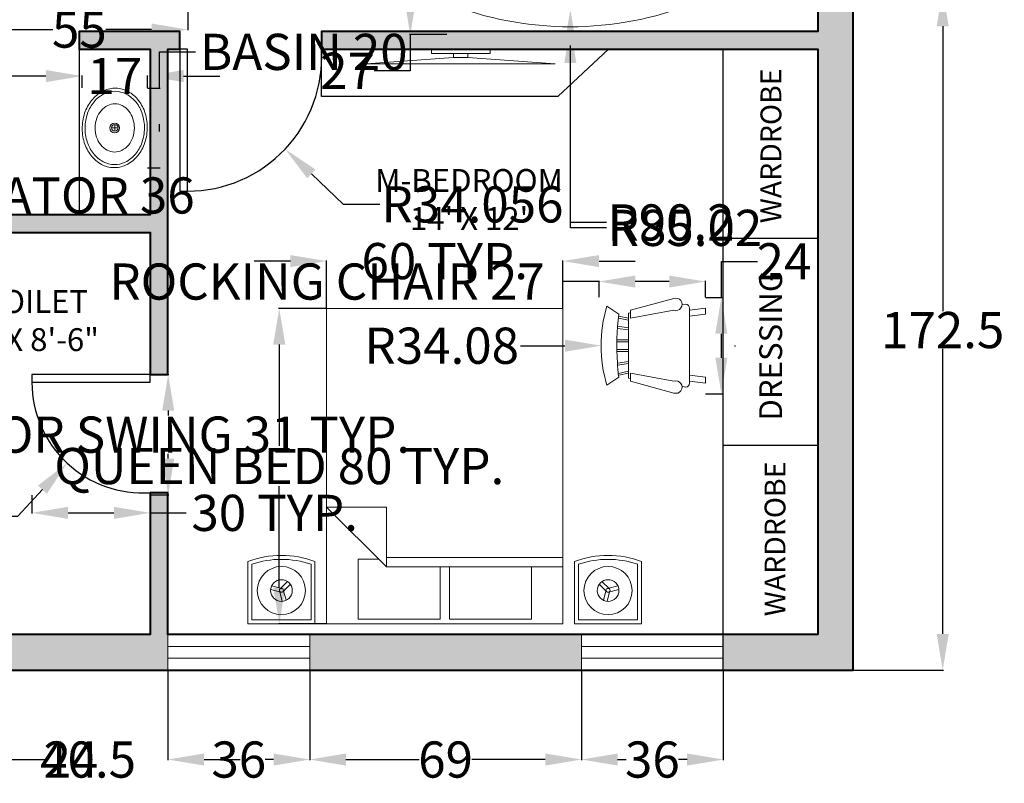
# Model space of a CAD drawing. Units: inches. Extents: x -51 to 563, y -59 to 453.
# Tile 4 of 6: x 211 to 461, y -59 to 134. Entities that reach past the tile are written whole.
import ezdxf

# ---------------------------------------------------------------- set-up
doc = ezdxf.new("R2010")
doc.units = ezdxf.units.IN
doc.header["$MEASUREMENT"] = 0
for name, color, linetype, lineweight in [('A-ANNO-DIMS', 2, 'Continuous', 18), ('A-ANNO-TEXT', 7, 'Continuous', 18), ('A-AREA-IDEN', 7, 'Continuous', 25), ('A-DOOR', 3, 'Continuous', 25), ('A-EQPM', 8, 'Continuous', 18), ('A-FLOR-CASE', 8, 'Continuous', 25), ('A-FLOR-FIXT', 9, 'Continuous', 18), ('A-FURN', 8, 'Continuous', 18), ('A-GLAZ', 4, 'Continuous', 18), ('A-WALL', 7, 'Continuous', 40), ('A-WALL-PATT', 252, 'Continuous', 13)]:
    doc.layers.add(name, color=color, linetype=linetype, lineweight=lineweight)
doc.styles.get("Standard").update_dxf_attribs({"font": 'arial.ttf'})
doc.dimstyles.get("Standard").update_dxf_attribs({"dimtxt": 9.18, "dimasz": 9.18, "dimexe": 0.18, "dimexo": 0.0625, "dimgap": 0.09, "dimtad": 0, "dimtih": 1, "dimtoh": 1, "dimdec": 1, "dimzin": 0, "dimdsep": 46, "dimlunit": 3, "dimtxsty": 'Standard', "dimcen": 0.09, "dimadec": 0, "dimazin": 0, "dimtfac": 1, "dimtdec": 1, "dimtofl": 0, "dimtmove": 0, "dimatfit": 3, "dimfxl": 1, "dimtolj": 1, "dimtzin": 0, "dimarcsym": 0})

# ---------------------------------------------------------------- blocks, each defined once
blk = doc.blocks.new('Bed - Queen')
for p, q in [((0, -80.00003), (0, 0)), ((0, 0), (59.99999, 0)), ((59.99999, 0), (59.99999, -80.00003)), ((7.99999, -1.2), (28.79998, -1.2)), ((7.99999, -14.4), (7.99999, -1.2)), ((28.79998, -1.2), (28.79998, -14.4)), ((31.19999, -1.2), (51.99999, -1.2)), ((31.19999, -14.4), (31.19999, -1.2)), ((51.99999, -1.2), (51.99999, -16.4)), ((0, -14.4), (44.8, -14.4)), ((59.99999, -29.6), (44.8, -14.4)), ((44.8, -14.4), (44.8, -29.6)), ((44.8, -16.8), (0, -16.8)), ((51.99999, -16.4), (46.79936, -16.4)), ((44.8, -29.6), (59.99999, -29.6)), ((59.99999, -80.00003), (0, -80.00003))]:
    blk.add_line(p, q)
blk = doc.blocks.new('Sink - Oval top')
for p, q in [((-1, 0), (1, 0)), ((0, 1), (0, -1))]:
    blk.add_line(p, q)
for points in [[(-12.23, 0.39, 0.117634), (-11.46, -3.36, 0.104469), (-8.88, -6.8, 0.090016), (-5.08, -9.07, 0.08192), (-0.32, -10.02, 0.08192), (4.49, -9.38, 0.090016), (8.42, -7.36, 0.104469), (11.22, -4.09, 0.117634), (12.23, -0.39, 0.117634), (11.46, 3.36, 0.104469), (8.88, 6.8, 0.090016), (5.08, 9.07, 0.08192), (0.32, 10.02, 0.08192), (-4.49, 9.38, 0.090016), (-8.42, 7.36, 0.104469), (-11.22, 4.09, 0.117634)], [(-11.29, 0.16, 0.118622), (-10.52, -3.25, 0.104678), (-8.07, -6.36, 0.089562), (-4.54, -8.37, 0.081185), (-0.13, -9.15, 0.081185), (4.3, -8.49, 0.089562), (7.89, -6.58, 0.104678), (10.42, -3.55, 0.118622), (11.29, -0.16, 0.118622), (10.52, 3.25, 0.104678), (8.07, 6.36, 0.089562), (4.54, 8.37, 0.081185), (0.13, 9.15, 0.081185), (-4.3, 8.49, 0.089562), (-7.89, 6.58, 0.104678), (-10.42, 3.55, 0.118622)], [(-7.42, 0.08, 0.118283), (-6.91, -2.17, 0.104607), (-5.29, -4.21, 0.089718), (-2.97, -5.53, 0.081436), (-0.07, -6.04, 0.081436), (2.84, -5.59, 0.089718), (5.2, -4.33, 0.104607), (6.86, -2.32, 0.118283), (7.42, -0.08, 0.118283), (6.91, 2.17, 0.104607), (5.29, 4.21, 0.089718), (2.97, 5.53, 0.081436), (0.07, 6.04, 0.081436), (-2.84, 5.59, 0.089718), (-5.2, 4.33, 0.104607), (-6.86, 2.32, 0.118283)]]:
    blk.add_lwpolyline(points, format="xyb", close=True)
for radius in [1.5, 1]:
    blk.add_circle((0, 0), radius)
blk = doc.blocks.new('Sofa - Roundback 7 ft.')
for p, q in [((-12.00002, -32.4421), (-12.00003, -6.5971)), ((11.99997, -32.4421), (11.99998, -6.5971)), ((-36.000027, -34), (-36.000027, -11.4696)), ((-35.999844, -13.3819), (35.9998, -13.3819)), ((35.99998, -34), (35.99998, -11.4696)), ((-36.000027, -32.4421), (35.99998, -32.4421))]:
    blk.add_line(p, q)
for points in [[(-36.000027, -34), (-42.000027, -34), (-42.000027, -8)], [(41.99998, -8), (41.99998, -34), (35.99998, -34)]]:
    blk.add_lwpolyline(points)
for centre, radius, start, end in [((0, -114.25), 114.25, 68.43141, 111.5686), ((-0.00001, -127.1968), 121.1968, 72.72033, 107.2797)]:
    blk.add_arc(centre, radius, start, end)
blk = doc.blocks.new('Chair - Rocking')
for p, q in [((-8, -4.5), (-10, -1.5)), ((8, -4.5), (10, -1.5)), ((-7.5, -4.5), (-7, -7)), ((-6.5, -7), (-7.02225, -4.43)), ((-4.5, -7), (-4.96674, -4.19951)), ((-4, -7), (-4.40532, -4.16272)), ((-1.5, -4.05012), (-1.5, -7)), ((-1, -7), (-1, -4.05012)), ((1, -7), (1, -4.04655)), ((1.5, -4.05012), (1.5, -7)), ((4, -7), (4.40187, -4.18694)), ((4.5, -7), (4.96761, -4.19437)), ((6.5, -7), (7, -4.4057)), ((7.5, -4.5), (7, -7)), ((-8.23428, -6.99939), (-8.3093, -7.47958)), ((-8.23041, -7), (8.23915, -7)), ((8.31071, -7.48854), (8.23449, -7.00073)), ((-9, -7.5), (-12, -18.49999)), ((-7, -7.5), (-9, -7.5)), ((-9, -18.49999), (-7, -7.5)), ((7, -7.5), (9, -7.5)), ((9, -18.49999), (7, -7.5)), ((9, -7.5), (12, -18.49999)), ((-10.36644, -20.64523), (-10.5, -21.49999)), ((10.5, -21.49999), (10.3575, -20.58798)), ((-9, -22.49999), (-9.5, -26.49999)), ((0, -22.49999), (-9.5, -22.49999)), ((-8, -26.49999), (-7.5, -22.49999)), ((0, -22.49999), (9.5, -22.49999)), ((8, -26.49999), (7.5, -22.49999)), ((9, -22.49999), (9.5, -26.49999)), ((-9.5, -26.49999), (-8, -26.49999)), ((9.5, -26.49999), (8, -26.49999))]:
    blk.add_line(p, q)
for centre, radius, start, end in [((0, -34.08333), 34.08333, 72.93847, 107.0615), ((0, -68.25004), 64.25, 93.92211, 97.15267), ((0, -68.25004), 64.25, 82.84733, 93.92211), ((-10.5, -18.99999), 1.58114, 161.5651, 18.43495), ((10.5, -18.99999), 1.58114, 161.5651, 18.43495), ((-9.5, -21.49999), 1, 180, 270), ((9.5, -21.49999), 1, 270, 0)]:
    blk.add_arc(centre, radius, start, end)
blk = doc.blocks.new('DR-SWING-30IN')
for p, q in [((30, 30.07), (0, 30.07)), ((0, 30.07), (0, 28.07)), ((30, 28.07), (30, 30.07)), ((0, 28.07), (30, 28.07))]:
    blk.add_line(p, q)
blk.add_arc((28.07, 28.07), 28.07, 180, 273.9499)
blk = doc.blocks.new('TV-FLATSCREEN-48IN')
for p, q in [((0, 0), (22.17, 1.61)), ((48, 0), (25.84, 1.61)), ((0, 0), (48, 0))]:
    blk.add_line(p, q)
for points in [[(16.55, 3.67), (31.46, 3.67), (31.46, 2.61), (16.55, 2.61)], [(22.17, 2.61), (25.84, 2.61), (25.84, 1.61), (22.17, 1.61)]]:
    blk.add_lwpolyline(points, close=True)
blk = doc.blocks.new('*U11')
for p, q in [((-1.31, -0.61), (0.61, 1.31)), ((-0.61, -1.31), (1.31, 0.61))]:
    blk.add_line(p, q)
blk = doc.blocks.new('*U12')
at = {"color": 0, "linetype": 'ByBlock', "lineweight": -2, "transparency": 16777216}
for p, rotation in [((276.07, -10.08), 120), ((277.73, -11.74), 239.9999999999999)]:
    blk.add_blockref('*U11', p, dxfattribs=dict(at, rotation=rotation))
blk.add_blockref('*U11', (278.34, -9.47), dxfattribs=at)
blk = doc.blocks.new('TABLE-SIDE-WITH-LAMP')
for points in [[(17.03, 15.79), (17.03, 0), (0, 0), (0, 15.79, -0.18199)], [(16.03, 15.08), (16.03, 1), (1, 1), (1, 15.08, -0.16668)]]:
    blk.add_lwpolyline(points, format="xyb", close=True)
for centre, radius in [((8.51, 8.42), 6.11), ((8.51, 8.42), 2.75), ((8.51, 8.47), 0.5)]:
    blk.add_circle(centre, radius)
blk.add_blockref('*U12', (-268.87, 18.9))
blk = doc.blocks.new('*D27')
at = {"layer": 'A-ANNO-DIMS', "color": 0, "lineweight": -2, "transparency": 16777216}
for p, q in [((288.78, 61.1), (276.66, 61.1)), ((276.84, 51.92), (276.84, 26.22)), ((276.84, -9.72), (276.84, 15.99)), ((288.78, -18.9), (276.66, -18.9))]:
    blk.add_line(p, q, dxfattribs=at)
at = {"layer": 'A-ANNO-DIMS', "color": 0, "transparency": 16777216}
for points in [[(275.31, 51.92), (278.37, 51.92), (276.84, 61.1)], [(275.31, -9.72), (278.37, -9.72), (276.84, -18.9)]]:
    blk.add_solid(points, dxfattribs=at)
at = {"layer": 'Defpoints', "color": 0, "transparency": 16777216}
for p in [(288.84, 61.1), (276.84, -18.9), (288.84, -18.9)]:
    blk.add_point(p, dxfattribs=at)
at = {"layer": 'A-ANNO-DIMS', "color": 0, "transparency": 16777216, "insert": (276.84, 21.1), "char_height": 9.18, "attachment_point": 5}
blk.add_mtext('\\A1;QUEEN BED 80 TYP.', dxfattribs=at)
blk = doc.blocks.new('*D28')
at = {"layer": 'A-ANNO-DIMS', "color": 0, "lineweight": -2, "transparency": 16777216}
for p, q in [((279.66, 73.1), (270.48, 73.1)), ((288.84, 61.17), (288.84, 73.28)), ((348.84, 61.17), (348.84, 73.28)), ((358.02, 73.1), (367.2, 73.1))]:
    blk.add_line(p, q, dxfattribs=at)
at = {"layer": 'A-ANNO-DIMS', "color": 0, "transparency": 16777216}
for points in [[(279.66, 74.63), (279.66, 71.57), (288.84, 73.1)], [(358.02, 74.63), (358.02, 71.57), (348.84, 73.1)]]:
    blk.add_solid(points, dxfattribs=at)
at = {"layer": 'Defpoints', "color": 0, "transparency": 16777216}
for p in [(288.84, 73.1), (288.84, 61.1), (348.84, 61.1)]:
    blk.add_point(p, dxfattribs=at)
at = {"layer": 'A-ANNO-DIMS', "color": 0, "transparency": 16777216, "insert": (318.84, 73.1), "char_height": 9.18, "attachment_point": 5}
blk.add_mtext('\\A1;60 TYP.', dxfattribs=at)
blk = doc.blocks.new('*D36')
at = {"layer": 'A-ANNO-DIMS', "color": 0, "lineweight": -2, "transparency": 16777216}
for p, q in [((319.42, 157.85), (309.92, 157.85)), ((310.1, 148.67), (310.1, 139.74)), ((319.42, 130.56), (309.92, 130.56)), ((310.1, 130.56), (310.1, 121.38)), ((310.1, 121.38), (300.92, 121.38))]:
    blk.add_line(p, q, dxfattribs=at)
at = {"layer": 'A-ANNO-DIMS', "color": 0, "transparency": 16777216}
for points in [[(308.57, 148.67), (311.63, 148.67), (310.1, 157.85)], [(308.57, 139.74), (311.63, 139.74), (310.1, 130.56)]]:
    blk.add_solid(points, dxfattribs=at)
at = {"layer": 'Defpoints', "color": 0, "transparency": 16777216}
for p in [(319.48, 157.85), (310.1, 130.56), (319.48, 130.56)]:
    blk.add_point(p, dxfattribs=at)
at = {"layer": 'A-ANNO-DIMS', "color": 0, "transparency": 16777216, "insert": (294.18, 121.38), "char_height": 9.18, "attachment_point": 5}
blk.add_mtext('\\A1;27', dxfattribs=at)
blk = doc.blocks.new('*D43')
at = {"layer": 'A-ANNO-DIMS', "color": 0, "lineweight": -2, "transparency": 16777216}
for p, q in [((244.12, 44.35), (248.82, 44.35)), ((248.64, 35.17), (248.64, 33.92)), ((248.64, 22.99), (248.64, 24.24)), ((244.12, 13.81), (248.82, 13.81))]:
    blk.add_line(p, q, dxfattribs=at)
at = {"layer": 'A-ANNO-DIMS', "color": 0, "transparency": 16777216}
for points in [[(247.11, 35.17), (250.17, 35.17), (248.64, 44.35)], [(247.11, 22.99), (250.17, 22.99), (248.64, 13.81)]]:
    blk.add_solid(points, dxfattribs=at)
at = {"layer": 'Defpoints', "color": 0, "transparency": 16777216}
for p in [(244.06, 44.35), (248.64, 44.35), (244.06, 13.81)]:
    blk.add_point(p, dxfattribs=at)
at = {"layer": 'A-ANNO-DIMS', "color": 0, "transparency": 16777216, "insert": (248.64, 29.08), "char_height": 9.18, "attachment_point": 5}
blk.add_mtext('\\A1;DOOR SWING 31 TYP.', dxfattribs=at)
blk = doc.blocks.new('*D44')
at = {"layer": 'A-ANNO-DIMS', "color": 0, "lineweight": -2, "transparency": 16777216}
for p, q in [((214.06, 13.75), (214.06, 9.05)), ((244.06, 13.75), (244.06, 9.05)), ((223.24, 9.23), (234.88, 9.23)), ((244.06, 9.23), (253.24, 9.23))]:
    blk.add_line(p, q, dxfattribs=at)
at = {"layer": 'A-ANNO-DIMS', "color": 0, "transparency": 16777216}
for points in [[(223.24, 10.76), (223.24, 7.7), (214.06, 9.23)], [(234.88, 10.76), (234.88, 7.7), (244.06, 9.23)]]:
    blk.add_solid(points, dxfattribs=at)
at = {"layer": 'Defpoints', "color": 0, "transparency": 16777216}
for p in [(214.06, 13.81), (244.06, 13.81), (244.06, 9.23)]:
    blk.add_point(p, dxfattribs=at)
at = {"layer": 'A-ANNO-DIMS', "color": 0, "transparency": 16777216, "insert": (275.67, 9.23), "char_height": 9.18, "attachment_point": 5}
blk.add_mtext('\\A1;30 TYP.', dxfattribs=at)
blk = doc.blocks.new('*D49')
at = {"layer": 'A-ANNO-DIMS', "color": 0, "lineweight": -2, "transparency": 16777216}
for p, q in [((246.41, 117), (246.41, 126.18)), ((246.41, 126.18), (255.59, 126.18)), ((243.43, 117), (246.59, 117)), ((246.41, 105.95), (246.41, 107.82)), ((243.43, 96.77), (246.59, 96.77))]:
    blk.add_line(p, q, dxfattribs=at)
at = {"layer": 'A-ANNO-DIMS', "color": 0, "transparency": 16777216}
for points in [[(244.88, 107.82), (247.94, 107.82), (246.41, 117)], [(244.88, 105.95), (247.94, 105.95), (246.41, 96.77)]]:
    blk.add_solid(points, dxfattribs=at)
at = {"layer": 'Defpoints', "color": 0, "transparency": 16777216}
for p in [(243.37, 117), (246.41, 117), (243.37, 96.77)]:
    blk.add_point(p, dxfattribs=at)
at = {"layer": 'A-ANNO-DIMS', "color": 0, "transparency": 16777216, "insert": (283.06, 126.18), "char_height": 9.18, "attachment_point": 5}
blk.add_mtext('\\A1;BASIN 20', dxfattribs=at)
blk = doc.blocks.new('*D50')
at = {"layer": 'A-ANNO-DIMS', "color": 0, "lineweight": -2, "transparency": 16777216}
for p, q in [((217.6, 120.04), (208.42, 120.04)), ((226.78, 117.06), (226.78, 120.22)), ((243.37, 117.06), (243.37, 120.22)), ((252.55, 120.04), (261.73, 120.04))]:
    blk.add_line(p, q, dxfattribs=at)
at = {"layer": 'A-ANNO-DIMS', "color": 0, "transparency": 16777216}
for points in [[(217.6, 121.57), (217.6, 118.51), (226.78, 120.04)], [(252.55, 121.57), (252.55, 118.51), (243.37, 120.04)]]:
    blk.add_solid(points, dxfattribs=at)
at = {"layer": 'Defpoints', "color": 0, "transparency": 16777216}
for p in [(226.78, 120.04), (226.78, 117), (243.37, 117)]:
    blk.add_point(p, dxfattribs=at)
at = {"layer": 'A-ANNO-DIMS', "color": 0, "transparency": 16777216, "insert": (235.08, 120.04), "char_height": 9.18, "attachment_point": 5}
blk.add_mtext('\\A1;17', dxfattribs=at)
blk = doc.blocks.new('*D55')
at = {"layer": 'A-ANNO-DIMS', "color": 0, "lineweight": -2, "transparency": 16777216}
for p, q in [((97.59, 95.09), (97.59, 89.57)), ((133.59, 95.09), (133.59, 89.57)), ((106.77, 89.75), (124.41, 89.75)), ((133.59, 89.75), (142.77, 89.75))]:
    blk.add_line(p, q, dxfattribs=at)
at = {"layer": 'A-ANNO-DIMS', "color": 0, "transparency": 16777216}
for points in [[(106.77, 91.28), (106.77, 88.22), (97.59, 89.75)], [(124.41, 91.28), (124.41, 88.22), (133.59, 89.75)]]:
    blk.add_solid(points, dxfattribs=at)
at = {"layer": 'Defpoints', "color": 0, "transparency": 16777216}
for p in [(97.59, 95.15), (133.59, 95.15), (133.59, 89.75)]:
    blk.add_point(p, dxfattribs=at)
at = {"layer": 'A-ANNO-DIMS', "color": 0, "transparency": 16777216, "insert": (201.92, 89.75), "char_height": 9.18, "attachment_point": 5}
blk.add_mtext('\\A1;REFRIGERATOR 36', dxfattribs=at)
blk = doc.blocks.new('*D58')
at = {"layer": 'A-ANNO-DIMS', "color": 0, "lineweight": -2, "transparency": 16777216}
for p, q in [((198.59, 145.43), (198.59, 131.66)), ((253.59, 145.43), (253.59, 131.66)), ((207.77, 131.84), (219.39, 131.84)), ((244.41, 131.84), (232.79, 131.84))]:
    blk.add_line(p, q, dxfattribs=at)
at = {"layer": 'A-ANNO-DIMS', "color": 0, "transparency": 16777216}
for points in [[(207.77, 133.37), (207.77, 130.31), (198.59, 131.84)], [(244.41, 133.37), (244.41, 130.31), (253.59, 131.84)]]:
    blk.add_solid(points, dxfattribs=at)
at = {"layer": 'Defpoints', "color": 0, "transparency": 16777216}
for p in [(198.59, 145.49), (253.59, 145.49), (253.59, 131.84)]:
    blk.add_point(p, dxfattribs=at)
at = {"layer": 'A-ANNO-DIMS', "color": 0, "transparency": 16777216, "insert": (226.09, 131.84), "char_height": 9.18, "attachment_point": 5}
blk.add_mtext('\\A1;55', dxfattribs=at)
blk = doc.blocks.new('*D63')
at = {"layer": 'A-ANNO-DIMS', "color": 0, "lineweight": -2, "transparency": 16777216}
for p, q in [((358.02, 67.91), (348.84, 67.91)), ((358.02, 63.92), (358.02, 68.09)), ((375.84, 67.91), (367.2, 67.91)), ((385.02, 63.92), (385.02, 68.09))]:
    blk.add_line(p, q, dxfattribs=at)
at = {"layer": 'A-ANNO-DIMS', "color": 0, "transparency": 16777216}
for points in [[(367.2, 69.44), (367.2, 66.38), (358.02, 67.91)], [(375.84, 69.44), (375.84, 66.38), (385.02, 67.91)]]:
    blk.add_solid(points, dxfattribs=at)
at = {"layer": 'Defpoints', "color": 0, "transparency": 16777216}
for p in [(358.02, 67.91), (358.02, 63.86), (385.02, 63.86)]:
    blk.add_point(p, dxfattribs=at)
at = {"layer": 'A-ANNO-DIMS', "color": 0, "transparency": 16777216, "insert": (288.97, 67.91), "char_height": 9.18, "attachment_point": 5}
blk.add_mtext('\\A1;ROCKING CHAIR 27', dxfattribs=at)
blk = doc.blocks.new('*D64')
at = {"layer": 'A-ANNO-DIMS', "color": 0, "lineweight": -2, "transparency": 16777216}
for p, q in [((389.07, 63.86), (389.07, 73.04)), ((389.07, 73.04), (398.25, 73.04)), ((385.08, 63.86), (389.25, 63.86)), ((389.07, 48.6), (389.07, 54.68)), ((385.08, 39.42), (389.25, 39.42))]:
    blk.add_line(p, q, dxfattribs=at)
at = {"layer": 'A-ANNO-DIMS', "color": 0, "transparency": 16777216}
for points in [[(387.54, 54.68), (390.6, 54.68), (389.07, 63.86)], [(387.54, 48.6), (390.6, 48.6), (389.07, 39.42)]]:
    blk.add_solid(points, dxfattribs=at)
at = {"layer": 'Defpoints', "color": 0, "transparency": 16777216}
for p in [(385.02, 63.86), (389.07, 63.86), (385.02, 39.42)]:
    blk.add_point(p, dxfattribs=at)
at = {"layer": 'A-ANNO-DIMS', "color": 0, "transparency": 16777216, "insert": (404.97, 73.04), "char_height": 9.18, "attachment_point": 5}
blk.add_mtext('\\A1;24', dxfattribs=at)
blk = doc.blocks.new('*D72')
at = {"layer": 'A-ANNO-DIMS', "color": 0, "lineweight": -2, "transparency": 16777216}
for p, q in [((422.62, 141.85), (445.44, 141.85)), ((445.26, 132.67), (445.26, 60.37)), ((445.26, -21.47), (445.26, 50.82)), ((422.62, -30.65), (445.44, -30.65))]:
    blk.add_line(p, q, dxfattribs=at)
at = {"layer": 'A-ANNO-DIMS', "color": 0, "transparency": 16777216}
for points in [[(443.73, 132.67), (446.79, 132.67), (445.26, 141.85)], [(443.73, -21.47), (446.79, -21.47), (445.26, -30.65)]]:
    blk.add_solid(points, dxfattribs=at)
at = {"layer": 'Defpoints', "color": 0, "transparency": 16777216}
for p in [(422.56, 141.85), (422.56, -30.65), (445.26, -30.65)]:
    blk.add_point(p, dxfattribs=at)
at = {"layer": 'A-ANNO-DIMS', "color": 0, "transparency": 16777216, "insert": (445.26, 55.6), "char_height": 9.18, "attachment_point": 5}
blk.add_mtext('\\A1;172.5', dxfattribs=at)
blk = doc.blocks.new('*D76')
at = {"layer": 'A-ANNO-DIMS', "color": 0, "lineweight": -2, "transparency": 16777216}
for p, q in [((184.06, -30.71), (184.06, -53.53)), ((208.06, -30.71), (208.06, -53.53)), ((193.24, -53.35), (198.88, -53.35)), ((208.06, -53.35), (217.24, -53.35))]:
    blk.add_line(p, q, dxfattribs=at)
at = {"layer": 'A-ANNO-DIMS', "color": 0, "transparency": 16777216}
for points in [[(193.24, -51.82), (193.24, -54.88), (184.06, -53.35)], [(198.88, -51.82), (198.88, -54.88), (208.06, -53.35)]]:
    blk.add_solid(points, dxfattribs=at)
at = {"layer": 'Defpoints', "color": 0, "transparency": 16777216}
for p in [(184.06, -30.65), (208.06, -30.65), (208.06, -53.35)]:
    blk.add_point(p, dxfattribs=at)
at = {"layer": 'A-ANNO-DIMS', "color": 0, "transparency": 16777216, "insert": (223.96, -53.35), "char_height": 9.18, "attachment_point": 5}
blk.add_mtext('\\A1;24', dxfattribs=at)
blk = doc.blocks.new('*D77')
at = {"layer": 'A-ANNO-DIMS', "color": 0, "lineweight": -2, "transparency": 16777216}
for p, q in [((208.058368, -30.714601), (208.058368, -53.532101)), ((248.558368, -30.714601), (248.558368, -53.532101)), ((198.878368, -53.352101), (189.698368, -53.352101)), ((257.738368, -53.352101), (266.918368, -53.352101))]:
    blk.add_line(p, q, dxfattribs=at)
at = {"layer": 'A-ANNO-DIMS', "color": 0, "transparency": 16777216}
for points in [[(198.878368, -51.822101), (198.878368, -54.882101), (208.058368, -53.352101)], [(257.738368, -51.822101), (257.738368, -54.882101), (248.558368, -53.352101)]]:
    blk.add_solid(points, dxfattribs=at)
at = {"layer": 'Defpoints', "color": 0, "transparency": 16777216}
for p in [(208.058368, -30.652101), (248.558368, -30.652101), (248.558368, -53.352101)]:
    blk.add_point(p, dxfattribs=at)
at = {"layer": 'A-ANNO-DIMS', "color": 0, "transparency": 16777216, "insert": (228.308368, -53.352101), "char_height": 9.18, "attachment_point": 5}
blk.add_mtext('\\A1;40.5', dxfattribs=at)
blk = doc.blocks.new('*D78')
at = {"layer": 'A-ANNO-DIMS', "color": 0, "lineweight": -2, "transparency": 16777216}
for p, q in [((248.56, -30.71), (248.56, -53.53)), ((284.56, -30.71), (284.56, -53.53)), ((257.74, -53.35), (259.9, -53.35)), ((275.38, -53.35), (273.22, -53.35))]:
    blk.add_line(p, q, dxfattribs=at)
at = {"layer": 'A-ANNO-DIMS', "color": 0, "transparency": 16777216}
for points in [[(257.74, -51.82), (257.74, -54.88), (248.56, -53.35)], [(275.38, -51.82), (275.38, -54.88), (284.56, -53.35)]]:
    blk.add_solid(points, dxfattribs=at)
at = {"layer": 'Defpoints', "color": 0, "transparency": 16777216}
for p in [(248.56, -30.65), (284.56, -30.65), (284.56, -53.35)]:
    blk.add_point(p, dxfattribs=at)
at = {"layer": 'A-ANNO-DIMS', "color": 0, "transparency": 16777216, "insert": (266.56, -53.35), "char_height": 9.18, "attachment_point": 5}
blk.add_mtext('\\A1;36', dxfattribs=at)
blk = doc.blocks.new('*D79')
at = {"layer": 'A-ANNO-DIMS', "color": 0, "lineweight": -2, "transparency": 16777216}
for p, q in [((284.56, -30.71), (284.56, -53.53)), ((353.56, -30.71), (353.56, -53.53)), ((293.74, -53.35), (312.36, -53.35)), ((344.38, -53.35), (325.76, -53.35))]:
    blk.add_line(p, q, dxfattribs=at)
at = {"layer": 'A-ANNO-DIMS', "color": 0, "transparency": 16777216}
for points in [[(293.74, -51.82), (293.74, -54.88), (284.56, -53.35)], [(344.38, -51.82), (344.38, -54.88), (353.56, -53.35)]]:
    blk.add_solid(points, dxfattribs=at)
at = {"layer": 'Defpoints', "color": 0, "transparency": 16777216}
for p in [(284.56, -30.65), (353.56, -30.65), (353.56, -53.35)]:
    blk.add_point(p, dxfattribs=at)
at = {"layer": 'A-ANNO-DIMS', "color": 0, "transparency": 16777216, "insert": (319.06, -53.35), "char_height": 9.18, "attachment_point": 5}
blk.add_mtext('\\A1;69', dxfattribs=at)
blk = doc.blocks.new('*D80')
at = {"layer": 'A-ANNO-DIMS', "color": 0, "lineweight": -2, "transparency": 16777216}
for p, q in [((353.56, -30.71), (353.56, -53.53)), ((389.56, -30.71), (389.56, -53.53)), ((362.74, -53.35), (364.9, -53.35)), ((380.38, -53.35), (378.22, -53.35))]:
    blk.add_line(p, q, dxfattribs=at)
at = {"layer": 'A-ANNO-DIMS', "color": 0, "transparency": 16777216}
for points in [[(362.74, -51.82), (362.74, -54.88), (353.56, -53.35)], [(380.38, -51.82), (380.38, -54.88), (389.56, -53.35)]]:
    blk.add_solid(points, dxfattribs=at)
at = {"layer": 'Defpoints', "color": 0, "transparency": 16777216}
for p in [(353.56, -30.65), (389.56, -30.65), (389.56, -53.35)]:
    blk.add_point(p, dxfattribs=at)
at = {"layer": 'A-ANNO-DIMS', "color": 0, "transparency": 16777216, "insert": (371.56, -53.35), "char_height": 9.18, "attachment_point": 5}
blk.add_mtext('\\A1;36', dxfattribs=at)
blk = doc.blocks.new('*D82')
at = {"layer": 'A-ANNO-DIMS', "color": 0, "lineweight": -2, "transparency": 16777216}
for p, q in [((253.56, 124.81), (253.56, 124.99)), ((253.47, 124.9), (253.65, 124.9)), ((293.17, 87.49), (284.99, 95.22)), ((302.35, 87.49), (293.17, 87.49))]:
    blk.add_line(p, q, dxfattribs=at)
at = {"layer": 'A-ANNO-DIMS', "color": 0, "transparency": 16777216}
blk.add_solid([(286.04, 96.33), (283.94, 94.1), (278.32, 101.52)], dxfattribs=at)
at = {"layer": 'Defpoints', "color": 0, "transparency": 16777216}
for p in [(253.56, 124.9), (278.32, 101.52)]:
    blk.add_point(p, dxfattribs=at)
at = {"layer": 'A-ANNO-DIMS', "color": 0, "transparency": 16777216, "insert": (325.89, 87.49), "char_height": 9.18, "attachment_point": 5}
blk.add_mtext('\\A1;R34.056', dxfattribs=at)
blk = doc.blocks.new('*D85')
at = {"layer": 'A-ANNO-DIMS', "color": 0, "lineweight": -2, "transparency": 16777216}
for p, q in [((242.04, 42.35), (242.22, 42.35)), ((242.13, 42.26), (242.13, 42.44)), ((210.45, 8.41), (216.71, 15.12)), ((201.27, 8.41), (210.45, 8.41))]:
    blk.add_line(p, q, dxfattribs=at)
at = {"layer": 'A-ANNO-DIMS', "color": 0, "transparency": 16777216}
blk.add_solid([(215.59, 16.16), (217.83, 14.07), (222.97, 21.83)], dxfattribs=at)
at = {"layer": 'Defpoints', "color": 0, "transparency": 16777216}
for p in [(242.13, 42.35), (222.97, 21.83)]:
    blk.add_point(p, dxfattribs=at)
at = {"layer": 'A-ANNO-DIMS', "color": 0, "transparency": 16777216, "insert": (167.79, 8.41), "char_height": 9.18, "attachment_point": 5}
blk.add_mtext('\\A1;2X R28.067', dxfattribs=at)
blk = doc.blocks.new('*D91')
at = {"layer": 'A-ANNO-DIMS', "color": 0, "lineweight": -2, "transparency": 16777216}
for p, q in [((350.65, 227.21), (350.83, 227.21)), ((350.74, 227.12), (350.74, 227.3)), ((350.74, 82.9), (350.74, 127.83)), ((359.92, 82.9), (350.74, 82.9))]:
    blk.add_line(p, q, dxfattribs=at)
at = {"layer": 'A-ANNO-DIMS', "color": 0, "transparency": 16777216}
blk.add_solid([(352.27, 127.83), (349.21, 127.83), (350.74, 137.01)], dxfattribs=at)
at = {"layer": 'Defpoints', "color": 0, "transparency": 16777216}
for p in [(350.74, 227.21), (350.74, 137.01)]:
    blk.add_point(p, dxfattribs=at)
at = {"layer": 'A-ANNO-DIMS', "color": 0, "transparency": 16777216, "insert": (376.27, 82.9), "char_height": 9.18, "attachment_point": 5}
blk.add_mtext('\\A1;R90.2', dxfattribs=at)
blk = doc.blocks.new('*D92')
at = {"layer": 'A-ANNO-DIMS', "color": 0, "lineweight": -2, "transparency": 16777216}
for p, q in [((350.65, 217.57), (350.83, 217.57)), ((350.74, 217.48), (350.74, 217.66)), ((350.74, 81.53), (350.74, 123.37)), ((359.92, 81.53), (350.74, 81.53))]:
    blk.add_line(p, q, dxfattribs=at)
at = {"layer": 'A-ANNO-DIMS', "color": 0, "transparency": 16777216}
blk.add_solid([(352.27, 123.37), (349.21, 123.37), (350.74, 132.55)], dxfattribs=at)
at = {"layer": 'Defpoints', "color": 0, "transparency": 16777216}
for p in [(350.74, 217.57), (350.74, 132.55)]:
    blk.add_point(p, dxfattribs=at)
at = {"layer": 'A-ANNO-DIMS', "color": 0, "transparency": 16777216, "insert": (379.84, 81.53), "char_height": 9.18, "attachment_point": 5}
blk.add_mtext('\\A1;R85.02', dxfattribs=at)
blk = doc.blocks.new('*D97')
at = {"layer": 'A-ANNO-DIMS', "color": 0, "lineweight": -2, "transparency": 16777216}
for p, q in [((338.07, 51.64), (349.34, 51.64)), ((392.51, 51.64), (392.69, 51.64)), ((392.6, 51.55), (392.6, 51.73))]:
    blk.add_line(p, q, dxfattribs=at)
at = {"layer": 'A-ANNO-DIMS', "color": 0, "transparency": 16777216}
blk.add_solid([(349.34, 53.17), (349.34, 50.11), (358.52, 51.64)], dxfattribs=at)
at = {"layer": 'Defpoints', "color": 0, "transparency": 16777216}
for p in [(358.52, 51.64), (392.6, 51.64)]:
    blk.add_point(p, dxfattribs=at)
at = {"layer": 'A-ANNO-DIMS', "color": 0, "transparency": 16777216, "insert": (318.09, 51.64), "char_height": 9.18, "attachment_point": 5}
blk.add_mtext('\\A1;R34.08', dxfattribs=at)

msp = doc.modelspace()

# ---------------------------------------------------------------- linework, layer by layer
at = {"layer": 'A-DOOR'}
for p, q in [((251.5584, 126.8479), (251.5584, 90.8479)), ((253.5584, 126.8479), (251.5584, 126.8479)), ((253.5584, 90.8479), (253.5584, 126.8479)), ((251.5584, 90.8479), (253.5584, 90.8479))]:
    msp.add_line(p, q, dxfattribs=at)
msp.add_arc((253.5584, 124.9035), 34.0556, 270, 3.273154, dxfattribs=at)
at = {"layer": 'A-FLOR-CASE'}
for p, q in [((226.0584, 126.8479), (226.0584, 84.8479)), ((287.5584, 114.8479), (287.5584, 126.8479)), ((347.5584, 114.8479), (360.3831, 126.8479)), ((389.5584, -30.6521), (389.5584, 126.8479))]:
    msp.add_line(p, q, dxfattribs=at)
for points in [[(347.5584, 114.8479), (287.5584, 114.8479)], [(413.5584, 78.8479), (389.5584, 78.8479)], [(413.5584, 26.3479), (389.5584, 26.3479)]]:
    msp.add_lwpolyline(points, dxfattribs=at)
at = {"layer": 'A-GLAZ'}
for p, q in [((248.5584, -21.6521), (248.5584, -30.6521)), ((284.5584, -21.6521), (284.5584, -30.6521)), ((353.5584, -30.6521), (353.5584, -21.6521))]:
    msp.add_line(p, q, dxfattribs=at)
for points in [[(284.5584, -24.6521), (248.5584, -24.6521)], [(389.5584, -24.6521), (353.5584, -24.6521)], [(284.5584, -27.6521), (248.5584, -27.6521)], [(389.5584, -27.6521), (353.5584, -27.6521)]]:
    msp.add_lwpolyline(points, dxfattribs=at)
at = {"layer": 'A-WALL'}
for points in [[(35.5584, -30.6521), (284.5584, -30.6521), (413.5584, -30.6521), (422.5584, -30.6521), (422.5584, 0.8479), (422.5584, 200.3479), (413.5584, 200.3479), (413.5584, 131.3479), (287.5584, 131.3479), (287.5584, 126.8479), (413.5584, 126.8479), (413.5584, -21.6521), (284.5584, -21.6521), (248.5584, -21.6521), (248.5584, 14.3479), (244.0584, 14.3479), (244.0584, -21.6521), (184.0584, -21.6521)], [(184.0584, 80.3479), (244.0584, 80.3479), (244.0584, 44.3479), (248.5584, 44.3479), (248.5584, 126.8479), (251.5584, 126.8479), (251.5584, 131.3479), (226.0584, 131.3479), (226.0584, 126.8479), (244.0584, 126.8479), (244.0584, 84.8479), (179.5584, 84.8479)]]:
    msp.add_lwpolyline(points, dxfattribs=at)
at = {"layer": 'A-WALL-PATT'}
for points in [[(413.5584, -21.6521), (422.5584, -30.6521), (413.5584, 141.8479), (422.5584, 141.8479)], [(251.5584, 126.8479), (251.5584, 131.3479), (226.0584, 126.8479), (226.0584, 131.3479)], [(244.0584, 126.8479), (248.5584, 126.8479), (251.5584, 126.8479), (251.5584, 131.3479)], [(413.5584, 126.8479), (413.5584, 131.3479), (287.5584, 126.8479), (287.5584, 131.3479)], [(244.0584, 44.3479), (248.5584, 44.3479), (244.0584, 126.8479), (248.5584, 126.8479)], [(184.0584, 80.3479), (179.5584, 84.8479), (244.0584, 80.3479), (244.0584, 84.8479)], [(244.0584, 80.3479), (244.0584, 84.8479), (244.0584, 44.3479), (248.5584, 44.3479)], [(244.0584, -21.6521), (248.5584, -30.6521), (244.0584, 14.3479), (248.5584, 14.3479)], [(208.0584, -21.6521), (208.0584, -30.6521), (244.0584, -21.6521), (248.5584, -30.6521)], [(284.5584, -21.6521), (284.5584, -30.6521), (353.5584, -21.6521), (353.5584, -30.6521)], [(389.5584, -21.6521), (389.5584, -30.6521), (413.5584, -21.6521), (422.5584, -30.6521)]]:
    msp.add_solid(points, dxfattribs=at)

# ---------------------------------------------------------------- block references
at = {"layer": 'A-DOOR'}
msp.add_blockref('DR-SWING-30IN', (214.058, 14.282), dxfattribs=at)
at = {"layer": 'A-EQPM'}
msp.add_blockref('TV-FLATSCREEN-48IN', (298.907, 123.175), dxfattribs=at)
at = {"layer": 'A-FLOR-FIXT', "xscale": 0.8240563005509539, "yscale": 0.8240563005509539, "zscale": 0.8240563005509539, "rotation": 90}
msp.add_blockref('Sink - Oval top', (235.0754, 106.8861), dxfattribs=at)
at = {"layer": 'A-FURN', "xscale": 0.7442004743752547, "yscale": 0.7442004743752547, "zscale": 0.7442004743752547, "rotation": 180}
msp.add_blockref('Sofa - Roundback 7 ft.', (350.7357, 132.5493), dxfattribs=at)
at = {"layer": 'A-FURN'}
for name, p, rotation in [('Chair - Rocking', (358.5179, 51.6377), 90), ('Bed - Queen', (348.8436, -18.8966), 180)]:
    msp.add_blockref(name, p, dxfattribs=dict(at, rotation=rotation))
msp.add_blockref('TABLE-SIDE-WITH-LAMP', (268.87, -18.897), dxfattribs=at)
at = {"layer": 'A-FURN', "extrusion": (0, 0, -1), "zscale": -1}
msp.add_blockref('TABLE-SIDE-WITH-LAMP', (-368.8172, -18.897), dxfattribs=at)

# ---------------------------------------------------------------- texts
at = {"layer": 'A-ANNO-TEXT', "char_height": 5.298513, "attachment_point": 1, "rotation": 90}
for insert in [(398.9999, 79.6901), (400.0507, -20.0339)]:
    msp.add_mtext_dynamic_manual_height_columns('\\pxqc;WARDROBE', width=45.301277, gutter_width=0.9135, heights=[0], dxfattribs=dict(at, insert=insert))
at = {"layer": 'A-AREA-IDEN', "char_height": 5.8, "attachment_point": 1}
for s, insert in [("\\pxqc;M-BEDROOM\\P14' X 12'", (300.2312, 96.454)), ('\\pxqc;TOILET\\P5\' X 8\'-6"', (190.204, 65.7447))]:
    msp.add_mtext_dynamic_manual_height_columns(s, width=49.588896, gutter_width=1, heights=[0], dxfattribs=dict(at, insert=insert))
at = {"layer": 'A-AREA-IDEN', "insert": (398.6913, 29.7461), "char_height": 5.8, "attachment_point": 1, "rotation": 90}
msp.add_mtext_dynamic_manual_height_columns('\\pxqc;DRESSING', width=43.815721, gutter_width=1, heights=[0], dxfattribs=at)

# ---------------------------------------------------------------- dimensions: what is measured, and where the dimension line sits
at = {"layer": 'A-ANNO-DIMS'}
for center, mpoint, override, picture, middle in [((350.7357, 227.2092), (350.736, 137.0145), {"dimdec": 1, "dimlfac": 1, "dimrnd": 0, "dimzin": 0, "dimdsep": 46, "dimlunit": 2}, '*D91', (376.2747, 82.8976)), ((350.7357, 217.5742), (350.736, 132.5493), {"dimdec": 2, "dimlfac": 1, "dimrnd": 0, "dimzin": 0, "dimdsep": 46, "dimlunit": 2}, '*D92', (379.8409, 81.5343)), ((253.5584, 124.9035), (278.3171, 101.5199), {"dimdec": 3, "dimlfac": 1, "dimrnd": 0, "dimzin": 0, "dimdsep": 46, "dimlunit": 2}, '*D82', (325.887, 87.4898)), ((392.6012, 51.6377), (358.5179, 51.638), {"dimdec": 2, "dimlfac": 1, "dimrnd": 0, "dimzin": 0, "dimdsep": 46, "dimlunit": 2}, '*D97', (338.0679, 51.6382))]:
    dim = msp.add_radius_dim(center=center, mpoint=mpoint, dimstyle='Standard', override=override, dxfattribs=at)
    dim.commit()
    dim.dimension.update_dxf_attribs({"geometry": picture, "text_midpoint": middle, "dimtype": 164})
for base, p1, p2, angle, override, picture, middle in [((310.1023, 130.5647), (319.4793, 157.8521), (319.4793, 130.5647), 270, {"dimdec": 0, "dimlfac": 1, "dimrnd": 0, "dimzin": 0, "dimdsep": 46, "dimlunit": 2}, '*D36', (294.179, 121.3847)), ((445.2584, -30.6521), (422.5584, 141.8479), (422.5584, -30.6521), 90, {"dimdec": 1, "dimlfac": 1, "dimrnd": 0, "dimzin": 0, "dimdsep": 46, "dimlunit": 2}, '*D72', (445.2584, 55.5979)), ((226.7786, 120.0365), (243.3723, 117.0018), (226.7786, 117.0018), 180, {"dimdec": 0, "dimlfac": 1, "dimrnd": 0, "dimzin": 0, "dimdsep": 46, "dimlunit": 2}, '*D50', (235.0754, 120.0365)), ((389.0679, 63.8552), (385.0179, 39.4201), (385.0179, 63.8552), 90, {"dimdec": 0, "dimlfac": 1, "dimrnd": 0, "dimzin": 0, "dimdsep": 46, "dimlunit": 2}, '*D64', (404.9724, 73.0352))]:
    dim = msp.add_linear_dim(base=base, p1=p1, p2=p2, angle=angle, dimstyle='Standard', override=override, dxfattribs=at)
    dim.commit()
    dim.dimension.update_dxf_attribs({"geometry": picture, "text_midpoint": middle})
for base, p1, p2, override, picture, middle in [((253.5874, 131.838), (198.5874, 145.488), (253.5874, 145.488), {"dimdec": 0, "dimlfac": 1, "dimrnd": 0, "dimzin": 0, "dimdsep": 46, "dimlunit": 2}, '*D58', (226.0874, 131.838)), ((208.0584, -53.3521), (184.0584, -30.6521), (208.0584, -30.6521), {"dimdec": 0, "dimlfac": 1, "dimrnd": 0, "dimzin": 0, "dimdsep": 46, "dimlunit": 2}, '*D76', (223.9629, -53.3521)), ((248.5584, -53.3521), (208.0584, -30.6521), (248.5584, -30.6521), {"dimdec": 1, "dimlfac": 1, "dimrnd": 0, "dimzin": 0, "dimdsep": 46, "dimlunit": 2}, '*D77', (228.3084, -53.3521)), ((284.5584, -53.3521), (248.5584, -30.6521), (284.5584, -30.6521), {"dimdec": 0, "dimlfac": 1, "dimrnd": 0, "dimzin": 0, "dimdsep": 46, "dimlunit": 2}, '*D78', (266.5584, -53.3521)), ((353.5584, -53.3521), (284.5584, -30.6521), (353.5584, -30.6521), {"dimdec": 0, "dimlfac": 1, "dimrnd": 0, "dimzin": 0, "dimdsep": 46, "dimlunit": 2}, '*D79', (319.0584, -53.3521)), ((389.5584, -53.3521), (353.5584, -30.6521), (389.5584, -30.6521), {"dimdec": 0, "dimlfac": 1, "dimrnd": 0, "dimzin": 0, "dimdsep": 46, "dimlunit": 2}, '*D80', (371.5584, -53.3521))]:
    dim = msp.add_linear_dim(base=base, p1=p1, p2=p2, dimstyle='Standard', override=override, dxfattribs=at)
    dim.commit()
    dim.dimension.update_dxf_attribs({"geometry": picture, "text_midpoint": middle})
for base, p1, p2, angle, text, picture, middle in [((246.407, 117.0018), (243.3723, 96.7705), (243.3723, 117.0018), 90, 'BASIN <>', '*D49', (283.0573, 126.1818)), ((358.0179, 67.9052), (385.0179, 63.8552), (358.0179, 63.8552), 180, 'ROCKING CHAIR <>', '*D63', (288.9715, 67.9052)), ((288.8436, 73.1034), (348.8436, 61.1034), (288.8436, 61.1034), 180, '<> TYP.', '*D28', (318.8436, 73.1034)), ((276.8436, -18.8966), (288.8436, 61.1034), (288.8436, -18.8966), 270, 'QUEEN BED <> TYP.', '*D27', (276.8436, 21.1034)), ((248.6388, 44.3479), (244.0584, 13.812), (244.0584, 44.3479), 90, 'DOOR SWING <> TYP.', '*D43', (248.6388, 29.08))]:
    dim = msp.add_linear_dim(base=base, p1=p1, p2=p2, angle=angle, text=text, dimstyle='Standard', override={"dimdec": 0, "dimlfac": 1, "dimrnd": 0, "dimzin": 0, "dimdsep": 46, "dimlunit": 2}, dxfattribs=at)
    dim.commit()
    dim.dimension.update_dxf_attribs({"geometry": picture, "text_midpoint": middle})
for base, p1, p2, text, picture, middle in [((133.5864, 89.7492), (97.5864, 95.1492), (133.5864, 95.1492), 'REFRIGERATOR <>', '*D55', (201.9159, 89.7492)), ((244.0584, 9.2316), (214.0584, 13.812), (244.0584, 13.812), '<> TYP.', '*D44', (275.6678, 9.2316))]:
    dim = msp.add_linear_dim(base=base, p1=p1, p2=p2, text=text, dimstyle='Standard', override={"dimdec": 0, "dimlfac": 1, "dimrnd": 0, "dimzin": 0, "dimdsep": 46, "dimlunit": 2}, dxfattribs=at)
    dim.commit()
    dim.dimension.update_dxf_attribs({"geometry": picture, "text_midpoint": middle})
dim = msp.add_radius_dim(center=(242.125, 42.3479), mpoint=(222.9746, 21.8296), text='2X <>', dimstyle='Standard', override={"dimdec": 3, "dimlfac": 1, "dimrnd": 0, "dimzin": 0, "dimdsep": 46, "dimlunit": 2}, dxfattribs=at)
dim.commit()
dim.dimension.update_dxf_attribs({"geometry": '*D85', "text_midpoint": (167.7886, 8.4074)})

doc.saveas('drawing.dxf')
